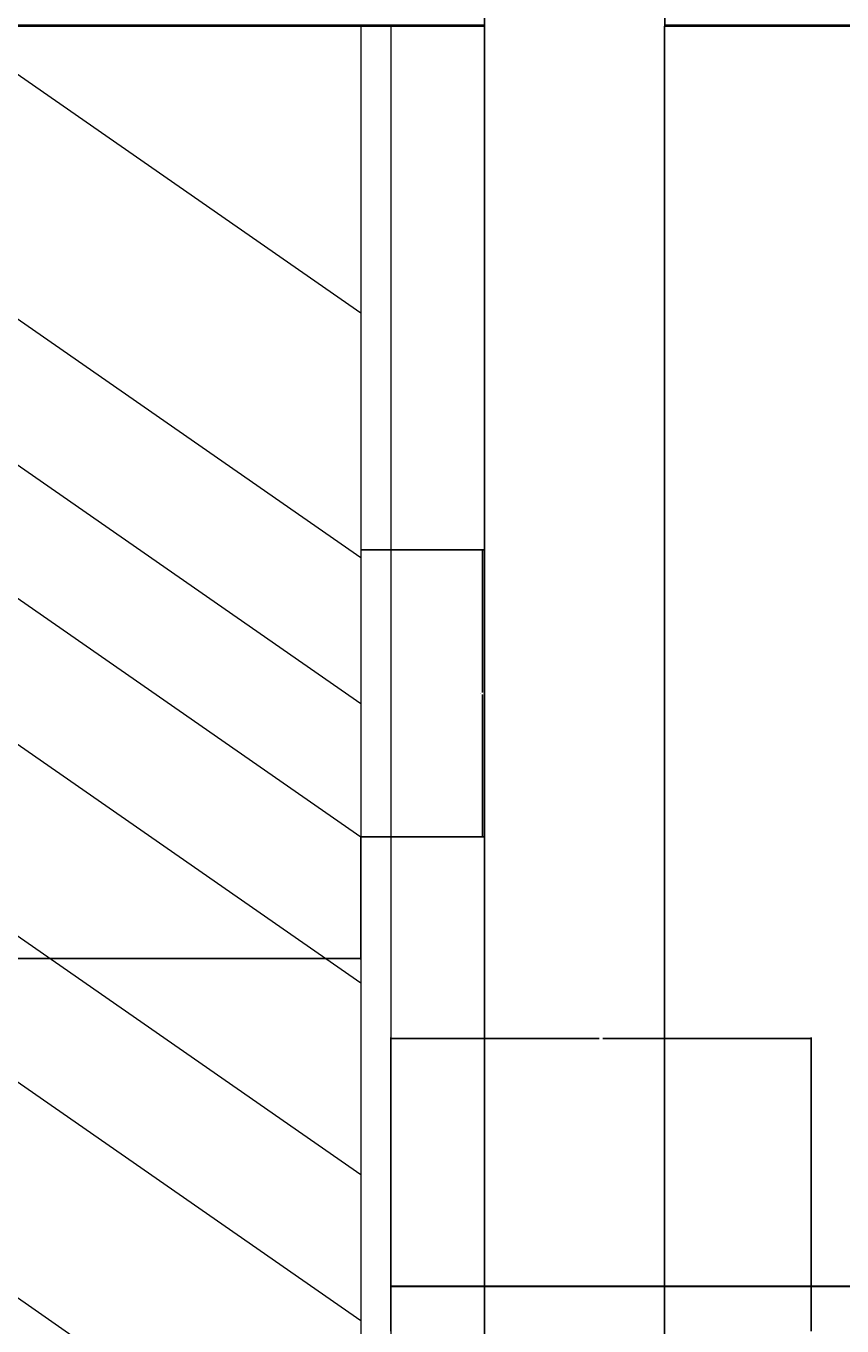
# Model space of a CAD drawing. Units: inches. Extents: x -46 to 1145, y -527 to 760.
# Tile 16 of 57: x 117 to 280, y -38 to 222. Entities that reach past the tile are written whole.
import ezdxf

# ---------------------------------------------------------------- set-up
doc = ezdxf.new("R2010")
doc.units = ezdxf.units.IN
doc.header["$MEASUREMENT"] = 0
for name, color, linetype, lineweight in [('A-ANNO-DIMS', 2, 'Continuous', 18), ('C-ROAD', 9, 'Continuous', 18), ('C-SITE', 7, 'Continuous', 30), ('DOORS', 3, 'Continuous', 25), ('WALLS', 4, 'Continuous', 40)]:
    doc.layers.add(name, color=color, linetype=linetype, lineweight=lineweight)
doc.styles.get("Standard").update_dxf_attribs({"font": 'arial.ttf'})
doc.dimstyles.get("Standard").update_dxf_attribs({"dimtxt": 0.18, "dimasz": 0.18, "dimexe": 0.18, "dimexo": 0.0625, "dimgap": 0.09, "dimtad": 0, "dimtih": 1, "dimtoh": 1, "dimdec": 0, "dimzin": 0, "dimdsep": 46, "dimlunit": 3, "dimtxsty": 'Standard', "dimcen": 0.09, "dimadec": 0, "dimazin": 0, "dimtfac": 1, "dimtdec": 0, "dimtofl": 0, "dimtmove": 0, "dimatfit": 3, "dimfxl": 1, "dimtolj": 1, "dimtzin": 0, "dimarcsym": 0})

# ---------------------------------------------------------------- blocks, each defined once
blk = doc.blocks.new('*U2')
for p, q in [((0, 0), (0, -6)), ((40, 0), (40, -6))]:
    blk.add_line(p, q)
blk.add_lwpolyline([(0, 0), (0, 40), (1.75, 40), (1.75, 0)], close=True)
blk.add_arc((0, 0), 40, 0, 90)
blk = doc.blocks.new('DRIVEWAY-CHEVRON')
for q in [(0, 2.03), (162, 0)]:
    blk.add_line((79.54, 57.38), q)
blk = doc.blocks.new('*D656')
at = {"layer": 'A-ANNO-DIMS', "color": 0, "lineweight": -2, "transparency": 16777216}
for p, q in [((21.56, 59.32), (21.56, 34.9)), ((183.56, 59.32), (183.56, 34.9)), ((21.74, 35.08), (100.93, 35.08)), ((183.38, 35.08), (104.2, 35.08))]:
    blk.add_line(p, q, dxfattribs=at)
at = {"layer": 'A-ANNO-DIMS', "color": 0, "transparency": 16777216}
for points in [[(21.74, 35.11), (21.74, 35.05), (21.56, 35.08)], [(183.38, 35.11), (183.38, 35.05), (183.56, 35.08)]]:
    blk.add_solid(points, dxfattribs=at)
at = {"layer": 'Defpoints', "color": 0, "transparency": 16777216}
for p in [(21.56, 59.38), (183.56, 59.38), (183.56, 35.08)]:
    blk.add_point(p, dxfattribs=at)
at = {"layer": 'A-ANNO-DIMS', "color": 0, "transparency": 16777216, "insert": (102.56, 35.08), "char_height": 0.18, "attachment_point": 5}
blk.add_mtext('\\A1;DRIVE MARKING 162 TYP.', dxfattribs=at)
blk = doc.blocks.new('*D657')
at = {"layer": 'A-ANNO-DIMS', "color": 0, "lineweight": -2, "transparency": 16777216}
for p, q in [((183.63, 116.76), (208.04, 116.76)), ((207.86, 116.58), (207.86, 88.25)), ((207.86, 59.56), (207.86, 87.89)), ((183.63, 59.38), (208.04, 59.38))]:
    blk.add_line(p, q, dxfattribs=at)
at = {"layer": 'A-ANNO-DIMS', "color": 0, "transparency": 16777216}
for points in [[(207.83, 116.58), (207.89, 116.58), (207.86, 116.76)], [(207.83, 59.56), (207.89, 59.56), (207.86, 59.38)]]:
    blk.add_solid(points, dxfattribs=at)
at = {"layer": 'Defpoints', "color": 0, "transparency": 16777216}
for p in [(183.56, 116.76), (207.86, 116.76), (183.56, 59.38)]:
    blk.add_point(p, dxfattribs=at)
at = {"layer": 'A-ANNO-DIMS', "color": 0, "transparency": 16777216, "insert": (207.86, 88.07), "char_height": 0.18, "attachment_point": 5}
blk.add_mtext('\\A1;57 TYP.', dxfattribs=at)
blk = doc.blocks.new('*D685')
at = {"layer": 'A-ANNO-DIMS', "color": 0, "lineweight": -2, "transparency": 16777216}
for p, q in [((183.5, 700.89), (-46.22, 700.89)), ((-46.04, 700.71), (-46.04, 116.39)), ((-46.04, -468.3), (-46.04, 116.02)), ((12.5, -468.48), (-46.22, -468.48))]:
    blk.add_line(p, q, dxfattribs=at)
at = {"layer": 'A-ANNO-DIMS', "color": 0, "transparency": 16777216}
for points in [[(-46.07, 700.71), (-46.01, 700.71), (-46.04, 700.89)], [(-46.07, -468.3), (-46.01, -468.3), (-46.04, -468.48)]]:
    blk.add_solid(points, dxfattribs=at)
at = {"layer": 'Defpoints', "color": 0, "transparency": 16777216}
for p in [(-46.04, 700.89), (183.56, 700.89), (12.56, -468.48)]:
    blk.add_point(p, dxfattribs=at)
at = {"layer": 'A-ANNO-DIMS', "color": 0, "transparency": 16777216, "insert": (-46.04, 116.2), "char_height": 0.18, "attachment_point": 5}
blk.add_mtext('\\A1;1169.4', dxfattribs=at)
blk = doc.blocks.new('*D693')
at = {"layer": 'A-ANNO-DIMS', "color": 0, "lineweight": -2, "transparency": 16777216}
for p, q in [((189.56, -39.42), (189.56, 19.3)), ((189.74, 19.12), (231.15, 19.12)), ((273.34, 19.12), (231.93, 19.12)), ((273.52, -39.42), (273.52, 19.3))]:
    blk.add_line(p, q, dxfattribs=at)
at = {"layer": 'A-ANNO-DIMS', "color": 0, "transparency": 16777216}
for points in [[(189.74, 19.15), (189.74, 19.09), (189.56, 19.12)], [(273.34, 19.15), (273.34, 19.09), (273.52, 19.12)]]:
    blk.add_solid(points, dxfattribs=at)
at = {"layer": 'Defpoints', "color": 0, "transparency": 16777216}
for p in [(273.52, 19.12), (189.56, -39.48), (273.52, -39.48)]:
    blk.add_point(p, dxfattribs=at)
at = {"layer": 'A-ANNO-DIMS', "color": 0, "transparency": 16777216, "insert": (231.54, 19.12), "char_height": 0.18, "attachment_point": 5}
blk.add_mtext('\\A1;83.95', dxfattribs=at)
blk = doc.blocks.new('*D695')
at = {"layer": 'A-ANNO-DIMS', "color": 0, "lineweight": -2, "transparency": 16777216}
for p, q in [((208.27, 221.46), (208.27, -527.26)), ((244.27, 221.46), (244.27, -527.26)), ((208.45, -527.08), (226.05, -527.08)), ((244.09, -527.08), (226.49, -527.08))]:
    blk.add_line(p, q, dxfattribs=at)
at = {"layer": 'A-ANNO-DIMS', "color": 0, "transparency": 16777216}
for points in [[(208.45, -527.05), (208.45, -527.11), (208.27, -527.08)], [(244.09, -527.05), (244.09, -527.11), (244.27, -527.08)]]:
    blk.add_solid(points, dxfattribs=at)
at = {"layer": 'Defpoints', "color": 0, "transparency": 16777216}
for p in [(208.27, 221.52), (244.27, 221.52), (244.27, -527.08)]:
    blk.add_point(p, dxfattribs=at)
at = {"layer": 'A-ANNO-DIMS', "color": 0, "transparency": 16777216, "insert": (226.27, -527.08), "char_height": 0.18, "attachment_point": 5}
blk.add_mtext('\\A1;36', dxfattribs=at)

msp = doc.modelspace()

# ---------------------------------------------------------------- linework, layer by layer
at = {"layer": 'C-ROAD'}
for p, q in [((183.5637, 221.5176), (183.5637, -459.4824)), ((189.5637, 221.5176), (189.5637, -468.4824))]:
    msp.add_line(p, q, dxfattribs=at)
at = {"layer": 'C-SITE'}
msp.add_line((590.0637, -30.4824), (189.5637, -30.4824), dxfattribs=at)
at = {"layer": 'WALLS'}
for p, q in [((208.2731, 221.5176), (12.5637, 221.5176)), ((509.0637, 221.5176), (244.2731, 221.5176))]:
    msp.add_line(p, q, dxfattribs=at)

# ---------------------------------------------------------------- block references
at = {"layer": 'C-ROAD'}
for p in [(21.564, 164.14), (21.564, 115.245), (21.564, 86.052), (21.564, 59.3801), (21.564, 30.1871), (21.564, -8.1106), (21.564, -37.3036), (21.564, -80.4757)]:
    msp.add_blockref('DRIVEWAY-CHEVRON', p, dxfattribs=at)
at = {"layer": 'DOORS', "xscale": 0.9, "yscale": 0.9, "zscale": 0.9}
msp.add_blockref('*U2', (208.2731, 226.9176), dxfattribs=at)

# ---------------------------------------------------------------- dimensions: what is measured, and where the dimension line sits
at = {"layer": 'A-ANNO-DIMS'}
dim = msp.add_linear_dim(base=(-46.0363, 700.8886), p1=(12.5637, -468.4824), p2=(183.5637, 700.8886), angle=90, dimstyle='Standard', override={"dimdec": 1, "dimlfac": 1, "dimrnd": 0, "dimzin": 0, "dimdsep": 46, "dimlunit": 2}, dxfattribs=at)
dim.commit()
dim.dimension.update_dxf_attribs({"geometry": '*D685', "text_midpoint": (-46.0363, 116.2031)})
for base, p1, p2, override, picture, middle in [((244.2731, -527.0824), (208.2731, 221.5176), (244.2731, 221.5176), {"dimdec": 0, "dimlfac": 1, "dimrnd": 0, "dimzin": 0, "dimdsep": 46, "dimlunit": 2}, '*D695', (226.2731, -527.0824)), ((273.5156, 19.1176), (189.5637, -39.4824), (273.5156, -39.4824), {"dimdec": 2, "dimlfac": 1, "dimrnd": 0, "dimzin": 0, "dimdsep": 46, "dimlunit": 2}, '*D693', (231.5397, 19.1176))]:
    dim = msp.add_linear_dim(base=base, p1=p1, p2=p2, dimstyle='Standard', override=override, dxfattribs=at)
    dim.commit()
    dim.dimension.update_dxf_attribs({"geometry": picture, "text_midpoint": middle})
dim = msp.add_linear_dim(base=(207.8637, 116.7577), p1=(183.5637, 59.3798), p2=(183.5637, 116.7577), angle=90, text='<> TYP.', dimstyle='Standard', override={"dimdec": 0, "dimlfac": 1, "dimrnd": 0, "dimzin": 0, "dimdsep": 46, "dimlunit": 2}, dxfattribs=at)
dim.commit()
dim.dimension.update_dxf_attribs({"geometry": '*D657', "text_midpoint": (207.8637, 88.0687)})
dim = msp.add_linear_dim(base=(183.5637, 35.0798), p1=(21.5637, 59.3798), p2=(183.5637, 59.3798), text='DRIVE MARKING <> TYP.', dimstyle='Standard', override={"dimdec": 0, "dimlfac": 1, "dimrnd": 0, "dimzin": 0, "dimdsep": 46, "dimlunit": 2}, dxfattribs=at)
dim.commit()
dim.dimension.update_dxf_attribs({"geometry": '*D656', "text_midpoint": (102.5637, 35.0798)})

doc.saveas('drawing.dxf')
